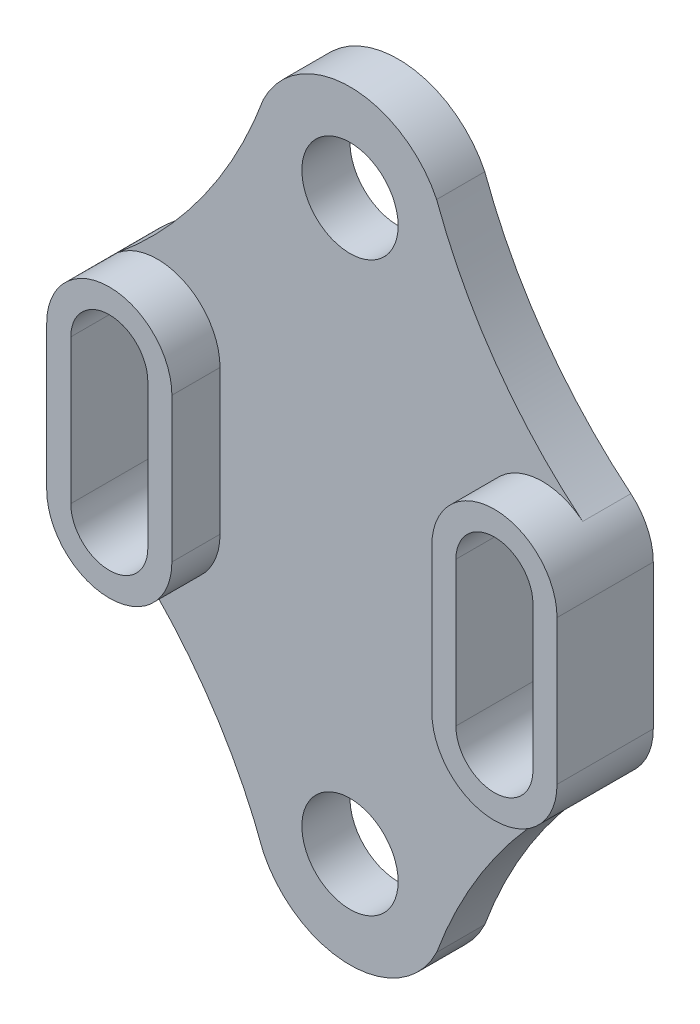
ISO-10303-21;
HEADER;
FILE_DESCRIPTION(('STEP AP214'),'2;1');
FILE_NAME('part.step','',(''),(''),'','','');
FILE_SCHEMA(('AUTOMOTIVE_DESIGN { 1 0 10303 214 1 1 1 1 }'));
ENDSEC;
DATA;
#1=APPLICATION_CONTEXT('core data for automotive mechanical design processes');
#2=APPLICATION_PROTOCOL_DEFINITION('international standard','automotive_design',2000,#1);
#3=PRODUCT_CONTEXT('',#1,'mechanical');
#4=PRODUCT('Part','Part','',(#3));
#5=PRODUCT_RELATED_PRODUCT_CATEGORY('part','',(#4));
#6=PRODUCT_DEFINITION_FORMATION('','',#4);
#7=PRODUCT_DEFINITION_CONTEXT('part definition',#1,'design');
#8=PRODUCT_DEFINITION('design','',#6,#7);
#9=PRODUCT_DEFINITION_SHAPE('','',#8);
#10=(LENGTH_UNIT() NAMED_UNIT(*) SI_UNIT(.MILLI.,.METRE.));
#11=(NAMED_UNIT(*) PLANE_ANGLE_UNIT() SI_UNIT($,.RADIAN.));
#12=(NAMED_UNIT(*) SI_UNIT($,.STERADIAN.) SOLID_ANGLE_UNIT());
#13=UNCERTAINTY_MEASURE_WITH_UNIT(LENGTH_MEASURE(1.E-05),#10,'distance_accuracy_value','');
#14=(GEOMETRIC_REPRESENTATION_CONTEXT(3) GLOBAL_UNCERTAINTY_ASSIGNED_CONTEXT((#13)) GLOBAL_UNIT_ASSIGNED_CONTEXT((#10,
#11,#12)) REPRESENTATION_CONTEXT('',''));
#15=CARTESIAN_POINT('',(0.,0.,0.));
#16=DIRECTION('',(0.,0.,1.));
#17=DIRECTION('',(1.,0.,0.));
#18=AXIS2_PLACEMENT_3D('',#15,#16,#17);
#19=CARTESIAN_POINT('',(0.,0.,10.));
#20=DIRECTION('',(0.,0.,1.));
#21=DIRECTION('',(1.,0.,0.));
#22=AXIS2_PLACEMENT_3D('',#19,#20,#21);
#23=PLANE('',#22);
#24=CARTESIAN_POINT('',(0.,-117.99999999991,10.));
#25=DIRECTION('',(0.,0.,1.));
#26=DIRECTION('',(1.,0.,0.));
#27=AXIS2_PLACEMENT_3D('',#24,#25,#26);
#28=CIRCLE('',#27,9.9999999999824);
#29=CARTESIAN_POINT('',(9.9999999999824,-117.99999999991,10.));
#30=VERTEX_POINT('',#29);
#31=EDGE_CURVE('E295',#30,#30,#28,.T.);
#32=ORIENTED_EDGE('',*,*,#31,.F.);
#33=EDGE_LOOP('',(#32));
#34=FACE_BOUND('',#33,.T.);
#35=CARTESIAN_POINT('',(0.,0.,10.));
#36=DIRECTION('',(0.,0.,1.));
#37=DIRECTION('',(1.,0.,0.));
#38=AXIS2_PLACEMENT_3D('',#35,#36,#37);
#39=CIRCLE('',#38,10.);
#40=CARTESIAN_POINT('',(10.,0.,10.));
#41=VERTEX_POINT('',#40);
#42=EDGE_CURVE('E301',#41,#41,#39,.T.);
#43=ORIENTED_EDGE('',*,*,#42,.F.);
#44=EDGE_LOOP('',(#43));
#45=FACE_BOUND('',#44,.T.);
#46=DIRECTION('',(0.,-1.,0.));
#47=VECTOR('',#46,1.);
#48=CARTESIAN_POINT('',(26.9999999996218,-43.9999999999274,10.));
#49=LINE('',#48,#47);
#50=CARTESIAN_POINT('',(26.9999999996218,-43.9999999999274,10.));
#51=VERTEX_POINT('',#50);
#52=CARTESIAN_POINT('',(26.9999999996218,-73.9999999999825,10.));
#53=VERTEX_POINT('',#52);
#54=EDGE_CURVE('E66',#51,#53,#49,.T.);
#55=ORIENTED_EDGE('',*,*,#54,.F.);
#56=CARTESIAN_POINT('',(39.9999999996218,-43.9999999999274,10.));
#57=DIRECTION('',(0.,0.,1.));
#58=DIRECTION('',(1.,0.,0.));
#59=AXIS2_PLACEMENT_3D('',#56,#57,#58);
#60=CIRCLE('',#59,13.);
#61=CARTESIAN_POINT('',(48.1941498448468,-33.9076311841338,10.));
#62=VERTEX_POINT('',#61);
#63=EDGE_CURVE('E255',#62,#51,#60,.T.);
#64=ORIENTED_EDGE('',*,*,#63,.F.);
#65=CARTESIAN_POINT('',(111.865980317354,43.2020180452665,10.));
#66=DIRECTION('',(0.,0.,1.));
#67=DIRECTION('',(1.,0.,0.));
#68=AXIS2_PLACEMENT_3D('',#65,#66,#67);
#69=CIRCLE('',#68,100.000000000004);
#70=CARTESIAN_POINT('',(17.9996405080933,8.71854010563166,10.));
#71=VERTEX_POINT('',#70);
#72=EDGE_CURVE('E386',#71,#62,#69,.T.);
#73=ORIENTED_EDGE('',*,*,#72,.F.);
#74=CARTESIAN_POINT('',(0.,0.,10.));
#75=DIRECTION('',(0.,0.,1.));
#76=DIRECTION('',(1.,0.,0.));
#77=AXIS2_PLACEMENT_3D('',#74,#75,#76);
#78=CIRCLE('',#77,19.9999999998526);
#79=CARTESIAN_POINT('',(-17.9996405080933,8.71854010563166,10.));
#80=VERTEX_POINT('',#79);
#81=EDGE_CURVE('E400',#71,#80,#78,.T.);
#82=ORIENTED_EDGE('',*,*,#81,.T.);
#83=CARTESIAN_POINT('',(-111.865980317354,43.2020180452665,10.));
#84=DIRECTION('',(0.,0.,1.));
#85=DIRECTION('',(1.,0.,0.));
#86=AXIS2_PLACEMENT_3D('',#83,#84,#85);
#87=CIRCLE('',#86,100.000000000004);
#88=CARTESIAN_POINT('',(-48.1941498448679,-33.9076311841512,10.));
#89=VERTEX_POINT('',#88);
#90=EDGE_CURVE('E360',#80,#89,#87,.F.);
#91=ORIENTED_EDGE('',*,*,#90,.T.);
#92=CARTESIAN_POINT('',(-39.9999999996218,-43.9999999999274,10.));
#93=DIRECTION('',(0.,0.,1.));
#94=DIRECTION('',(1.,0.,0.));
#95=AXIS2_PLACEMENT_3D('',#92,#93,#94);
#96=CIRCLE('',#95,13.);
#97=CARTESIAN_POINT('',(-26.9999999996218,-43.9999999999274,10.));
#98=VERTEX_POINT('',#97);
#99=EDGE_CURVE('E316',#98,#89,#96,.T.);
#100=ORIENTED_EDGE('',*,*,#99,.F.);
#101=DIRECTION('',(0.,1.,0.));
#102=VECTOR('',#101,1.);
#103=CARTESIAN_POINT('',(-26.9999999996218,-43.9999999999274,10.));
#104=LINE('',#103,#102);
#105=CARTESIAN_POINT('',(-26.9999999996218,-73.9999999999825,10.));
#106=VERTEX_POINT('',#105);
#107=EDGE_CURVE('E321',#106,#98,#104,.T.);
#108=ORIENTED_EDGE('',*,*,#107,.F.);
#109=CARTESIAN_POINT('',(-39.9999999996218,-73.9999999999825,10.));
#110=DIRECTION('',(0.,0.,1.));
#111=DIRECTION('',(1.,0.,0.));
#112=AXIS2_PLACEMENT_3D('',#109,#110,#111);
#113=CIRCLE('',#112,13.);
#114=CARTESIAN_POINT('',(-48.1941498448539,-84.0923688157703,10.));
#115=VERTEX_POINT('',#114);
#116=EDGE_CURVE('E11',#115,#106,#113,.T.);
#117=ORIENTED_EDGE('',*,*,#116,.F.);
#118=CARTESIAN_POINT('',(-111.865980317354,-161.202018045176,10.));
#119=DIRECTION('',(0.,0.,1.));
#120=DIRECTION('',(1.,0.,0.));
#121=AXIS2_PLACEMENT_3D('',#118,#119,#120);
#122=CIRCLE('',#121,100.000000000004);
#123=CARTESIAN_POINT('',(-17.9996405080933,-126.718540105542,10.));
#124=VERTEX_POINT('',#123);
#125=EDGE_CURVE('E459',#124,#115,#122,.T.);
#126=ORIENTED_EDGE('',*,*,#125,.F.);
#127=CARTESIAN_POINT('',(0.,-117.99999999991,10.));
#128=DIRECTION('',(0.,0.,1.));
#129=DIRECTION('',(1.,0.,0.));
#130=AXIS2_PLACEMENT_3D('',#127,#128,#129);
#131=CIRCLE('',#130,19.9999999998526);
#132=CARTESIAN_POINT('',(17.9996405080933,-126.718540105542,10.));
#133=VERTEX_POINT('',#132);
#134=EDGE_CURVE('E520',#124,#133,#131,.T.);
#135=ORIENTED_EDGE('',*,*,#134,.T.);
#136=CARTESIAN_POINT('',(111.865980317354,-161.202018045176,10.));
#137=DIRECTION('',(0.,0.,1.));
#138=DIRECTION('',(1.,0.,0.));
#139=AXIS2_PLACEMENT_3D('',#136,#137,#138);
#140=CIRCLE('',#139,100.000000000004);
#141=CARTESIAN_POINT('',(48.1941498448468,-84.0923688157761,10.));
#142=VERTEX_POINT('',#141);
#143=EDGE_CURVE('E397',#133,#142,#140,.F.);
#144=ORIENTED_EDGE('',*,*,#143,.T.);
#145=CARTESIAN_POINT('',(39.9999999996218,-73.9999999999825,10.));
#146=DIRECTION('',(0.,0.,1.));
#147=DIRECTION('',(1.,0.,0.));
#148=AXIS2_PLACEMENT_3D('',#145,#146,#147);
#149=CIRCLE('',#148,13.);
#150=EDGE_CURVE('E72',#53,#142,#149,.T.);
#151=ORIENTED_EDGE('',*,*,#150,.F.);
#152=EDGE_LOOP('',(#55,#64,#73,#82,#91,#100,#108,#117,#126,#135,#144,#151));
#153=FACE_BOUND('',#152,.T.);
#154=ADVANCED_FACE('F50',(#34,#45,#153),#23,.T.);
#155=CARTESIAN_POINT('',(0.,-117.99999999991,10.));
#156=DIRECTION('',(0.,0.,-1.));
#157=DIRECTION('',(-1.,0.,0.));
#158=AXIS2_PLACEMENT_3D('',#155,#156,#157);
#159=CYLINDRICAL_SURFACE('',#158,19.9999999998526);
#160=CARTESIAN_POINT('',(0.,-117.99999999991,0.));
#161=DIRECTION('',(0.,0.,1.));
#162=DIRECTION('',(1.,0.,0.));
#163=AXIS2_PLACEMENT_3D('',#160,#161,#162);
#164=CIRCLE('',#163,19.9999999998526);
#165=CARTESIAN_POINT('',(-17.9996405080933,-126.718540105542,0.));
#166=VERTEX_POINT('',#165);
#167=CARTESIAN_POINT('',(17.9996405080933,-126.718540105542,0.));
#168=VERTEX_POINT('',#167);
#169=EDGE_CURVE('E526',#166,#168,#164,.T.);
#170=ORIENTED_EDGE('',*,*,#169,.T.);
#171=DIRECTION('',(0.,0.,-1.));
#172=VECTOR('',#171,1.);
#173=CARTESIAN_POINT('',(17.9996405080933,-126.718540105542,10.));
#174=LINE('',#173,#172);
#175=EDGE_CURVE('E59',#133,#168,#174,.T.);
#176=ORIENTED_EDGE('',*,*,#175,.F.);
#177=ORIENTED_EDGE('',*,*,#134,.F.);
#178=DIRECTION('',(0.,0.,-1.));
#179=VECTOR('',#178,1.);
#180=CARTESIAN_POINT('',(-17.9996405080933,-126.718540105542,10.));
#181=LINE('',#180,#179);
#182=EDGE_CURVE('E464',#124,#166,#181,.T.);
#183=ORIENTED_EDGE('',*,*,#182,.T.);
#184=EDGE_LOOP('',(#170,#176,#177,#183));
#185=FACE_BOUND('',#184,.T.);
#186=ADVANCED_FACE('F47',(#185),#159,.T.);
#187=CARTESIAN_POINT('',(111.865980317354,-161.202018045176,10.));
#188=DIRECTION('',(0.,0.,-1.));
#189=DIRECTION('',(-1.,0.,0.));
#190=AXIS2_PLACEMENT_3D('',#187,#188,#189);
#191=CYLINDRICAL_SURFACE('',#190,100.000000000004);
#192=CARTESIAN_POINT('',(111.865980317354,-161.202018045176,0.));
#193=DIRECTION('',(0.,0.,1.));
#194=DIRECTION('',(1.,0.,0.));
#195=AXIS2_PLACEMENT_3D('',#192,#193,#194);
#196=CIRCLE('',#195,100.000000000004);
#197=CARTESIAN_POINT('',(48.341000131319,-83.971344784064,0.));
#198=VERTEX_POINT('',#197);
#199=EDGE_CURVE('E529',#168,#198,#196,.F.);
#200=ORIENTED_EDGE('',*,*,#199,.T.);
#201=DIRECTION('',(0.,0.,-1.));
#202=VECTOR('',#201,1.);
#203=CARTESIAN_POINT('',(48.341000131319,-83.971344784064,10.));
#204=LINE('',#203,#202);
#205=CARTESIAN_POINT('',(48.341000131319,-83.971344784064,10.));
#206=VERTEX_POINT('',#205);
#207=EDGE_CURVE('E440',#206,#198,#204,.T.);
#208=ORIENTED_EDGE('',*,*,#207,.F.);
#209=CARTESIAN_POINT('',(39.9999999996218,-73.9999999999825,10.));
#210=DIRECTION('',(0.,0.,1.));
#211=DIRECTION('',(0.630319218863457,-0.776336062753342,0.));
#212=AXIS2_PLACEMENT_3D('',#209,#210,#211);
#213=CIRCLE('',#212,13.);
#214=EDGE_CURVE('E287',#142,#206,#213,.T.);
#215=ORIENTED_EDGE('',*,*,#214,.F.);
#216=ORIENTED_EDGE('',*,*,#143,.F.);
#217=ORIENTED_EDGE('',*,*,#175,.T.);
#218=EDGE_LOOP('',(#200,#208,#215,#216,#217));
#219=FACE_BOUND('',#218,.T.);
#220=ADVANCED_FACE('F412',(#219),#191,.F.);
#221=CARTESIAN_POINT('',(39.9999999996218,-73.9999999999825,10.));
#222=DIRECTION('',(0.,0.,-1.));
#223=DIRECTION('',(-1.,0.,0.));
#224=AXIS2_PLACEMENT_3D('',#221,#222,#223);
#225=CYLINDRICAL_SURFACE('',#224,13.);
#226=CARTESIAN_POINT('',(39.9999999996218,-73.9999999999825,0.));
#227=DIRECTION('',(0.,0.,1.));
#228=DIRECTION('',(1.,0.,0.));
#229=AXIS2_PLACEMENT_3D('',#226,#227,#228);
#230=CIRCLE('',#229,13.);
#231=CARTESIAN_POINT('',(52.9999999996218,-73.9999999999825,0.));
#232=VERTEX_POINT('',#231);
#233=EDGE_CURVE('E535',#198,#232,#230,.T.);
#234=ORIENTED_EDGE('',*,*,#233,.T.);
#235=DIRECTION('',(0.,0.,-1.));
#236=VECTOR('',#235,1.);
#237=CARTESIAN_POINT('',(52.9999999996218,-73.9999999999825,10.));
#238=LINE('',#237,#236);
#239=CARTESIAN_POINT('',(52.9999999996218,-73.9999999999825,20.));
#240=VERTEX_POINT('',#239);
#241=EDGE_CURVE('E437',#240,#232,#238,.T.);
#242=ORIENTED_EDGE('',*,*,#241,.F.);
#243=CARTESIAN_POINT('',(39.9999999996218,-73.9999999999825,20.));
#244=DIRECTION('',(0.,0.,1.));
#245=DIRECTION('',(1.,0.,0.));
#246=AXIS2_PLACEMENT_3D('',#243,#244,#245);
#247=CIRCLE('',#246,13.);
#248=CARTESIAN_POINT('',(26.9999999996218,-73.9999999999825,20.));
#249=VERTEX_POINT('',#248);
#250=EDGE_CURVE('E257',#249,#240,#247,.T.);
#251=ORIENTED_EDGE('',*,*,#250,.F.);
#252=DIRECTION('',(0.,0.,-1.));
#253=VECTOR('',#252,1.);
#254=CARTESIAN_POINT('',(26.9999999996218,-73.9999999999825,20.));
#255=LINE('',#254,#253);
#256=EDGE_CURVE('E266',#249,#53,#255,.T.);
#257=ORIENTED_EDGE('',*,*,#256,.T.);
#258=ORIENTED_EDGE('',*,*,#150,.T.);
#259=ORIENTED_EDGE('',*,*,#214,.T.);
#260=ORIENTED_EDGE('',*,*,#207,.T.);
#261=EDGE_LOOP('',(#234,#242,#251,#257,#258,#259,#260));
#262=FACE_BOUND('',#261,.T.);
#263=ADVANCED_FACE('F425',(#262),#225,.T.);
#264=CARTESIAN_POINT('',(52.9999999996218,0.,10.));
#265=DIRECTION('',(-1.,0.,0.));
#266=DIRECTION('',(0.,-1.,0.));
#267=AXIS2_PLACEMENT_3D('',#264,#265,#266);
#268=PLANE('',#267);
#269=DIRECTION('',(0.,1.,0.));
#270=VECTOR('',#269,1.);
#271=CARTESIAN_POINT('',(52.9999999996218,0.,0.));
#272=LINE('',#271,#270);
#273=CARTESIAN_POINT('',(52.9999999996218,-43.9999999999274,0.));
#274=VERTEX_POINT('',#273);
#275=EDGE_CURVE('E506',#232,#274,#272,.T.);
#276=ORIENTED_EDGE('',*,*,#275,.T.);
#277=DIRECTION('',(0.,0.,-1.));
#278=VECTOR('',#277,1.);
#279=CARTESIAN_POINT('',(52.9999999996218,-43.9999999999274,10.));
#280=LINE('',#279,#278);
#281=CARTESIAN_POINT('',(52.9999999996218,-43.9999999999274,20.));
#282=VERTEX_POINT('',#281);
#283=EDGE_CURVE('E401',#282,#274,#280,.T.);
#284=ORIENTED_EDGE('',*,*,#283,.F.);
#285=DIRECTION('',(0.,1.,0.));
#286=VECTOR('',#285,1.);
#287=CARTESIAN_POINT('',(52.9999999996218,-73.9999999999825,20.));
#288=LINE('',#287,#286);
#289=EDGE_CURVE('E263',#240,#282,#288,.T.);
#290=ORIENTED_EDGE('',*,*,#289,.F.);
#291=ORIENTED_EDGE('',*,*,#241,.T.);
#292=EDGE_LOOP('',(#276,#284,#290,#291));
#293=FACE_BOUND('',#292,.T.);
#294=ADVANCED_FACE('F422',(#293),#268,.F.);
#295=CARTESIAN_POINT('',(39.9999999996218,-43.9999999999274,10.));
#296=DIRECTION('',(0.,0.,-1.));
#297=DIRECTION('',(-1.,0.,0.));
#298=AXIS2_PLACEMENT_3D('',#295,#296,#297);
#299=CYLINDRICAL_SURFACE('',#298,13.);
#300=CARTESIAN_POINT('',(39.9999999996218,-43.9999999999274,0.));
#301=DIRECTION('',(0.,0.,1.));
#302=DIRECTION('',(1.,0.,0.));
#303=AXIS2_PLACEMENT_3D('',#300,#301,#302);
#304=CIRCLE('',#303,13.);
#305=CARTESIAN_POINT('',(48.341000131319,-34.0286552158459,0.));
#306=VERTEX_POINT('',#305);
#307=EDGE_CURVE('E501',#274,#306,#304,.T.);
#308=ORIENTED_EDGE('',*,*,#307,.T.);
#309=DIRECTION('',(0.,0.,-1.));
#310=VECTOR('',#309,1.);
#311=CARTESIAN_POINT('',(48.341000131319,-34.0286552158459,10.));
#312=LINE('',#311,#310);
#313=CARTESIAN_POINT('',(48.341000131319,-34.0286552158459,10.));
#314=VERTEX_POINT('',#313);
#315=EDGE_CURVE('E402',#314,#306,#312,.T.);
#316=ORIENTED_EDGE('',*,*,#315,.F.);
#317=CARTESIAN_POINT('',(39.9999999996218,-43.9999999999274,10.));
#318=DIRECTION('',(0.,0.,1.));
#319=DIRECTION('',(0.641615394745934,0.767026521852419,0.));
#320=AXIS2_PLACEMENT_3D('',#317,#318,#319);
#321=CIRCLE('',#320,13.);
#322=EDGE_CURVE('E281',#314,#62,#321,.T.);
#323=ORIENTED_EDGE('',*,*,#322,.T.);
#324=ORIENTED_EDGE('',*,*,#63,.T.);
#325=DIRECTION('',(0.,0.,-1.));
#326=VECTOR('',#325,1.);
#327=CARTESIAN_POINT('',(26.9999999996218,-43.9999999999274,20.));
#328=LINE('',#327,#326);
#329=CARTESIAN_POINT('',(26.9999999996218,-43.9999999999274,20.));
#330=VERTEX_POINT('',#329);
#331=EDGE_CURVE('E272',#330,#51,#328,.T.);
#332=ORIENTED_EDGE('',*,*,#331,.F.);
#333=CARTESIAN_POINT('',(39.9999999996218,-43.9999999999274,20.));
#334=DIRECTION('',(0.,0.,1.));
#335=DIRECTION('',(1.,0.,0.));
#336=AXIS2_PLACEMENT_3D('',#333,#334,#335);
#337=CIRCLE('',#336,13.);
#338=EDGE_CURVE('E254',#282,#330,#337,.T.);
#339=ORIENTED_EDGE('',*,*,#338,.F.);
#340=ORIENTED_EDGE('',*,*,#283,.T.);
#341=EDGE_LOOP('',(#308,#316,#323,#324,#332,#339,#340));
#342=FACE_BOUND('',#341,.T.);
#343=ADVANCED_FACE('F377',(#342),#299,.T.);
#344=CARTESIAN_POINT('',(111.865980317354,43.2020180452665,10.));
#345=DIRECTION('',(0.,0.,-1.));
#346=DIRECTION('',(-1.,0.,0.));
#347=AXIS2_PLACEMENT_3D('',#344,#345,#346);
#348=CYLINDRICAL_SURFACE('',#347,100.000000000004);
#349=CARTESIAN_POINT('',(111.865980317354,43.2020180452665,0.));
#350=DIRECTION('',(0.,0.,1.));
#351=DIRECTION('',(1.,0.,0.));
#352=AXIS2_PLACEMENT_3D('',#349,#350,#351);
#353=CIRCLE('',#352,100.000000000004);
#354=CARTESIAN_POINT('',(17.9996405080933,8.71854010563166,0.));
#355=VERTEX_POINT('',#354);
#356=EDGE_CURVE('E496',#355,#306,#353,.T.);
#357=ORIENTED_EDGE('',*,*,#356,.F.);
#358=DIRECTION('',(0.,0.,-1.));
#359=VECTOR('',#358,1.);
#360=CARTESIAN_POINT('',(17.9996405080933,8.71854010563166,10.));
#361=LINE('',#360,#359);
#362=EDGE_CURVE('E404',#71,#355,#361,.T.);
#363=ORIENTED_EDGE('',*,*,#362,.F.);
#364=ORIENTED_EDGE('',*,*,#72,.T.);
#365=ORIENTED_EDGE('',*,*,#322,.F.);
#366=ORIENTED_EDGE('',*,*,#315,.T.);
#367=EDGE_LOOP('',(#357,#363,#364,#365,#366));
#368=FACE_BOUND('',#367,.T.);
#369=ADVANCED_FACE('F374',(#368),#348,.F.);
#370=CARTESIAN_POINT('',(0.,0.,10.));
#371=DIRECTION('',(0.,0.,-1.));
#372=DIRECTION('',(-1.,0.,0.));
#373=AXIS2_PLACEMENT_3D('',#370,#371,#372);
#374=CYLINDRICAL_SURFACE('',#373,19.9999999998526);
#375=CARTESIAN_POINT('',(0.,0.,0.));
#376=DIRECTION('',(0.,0.,1.));
#377=DIRECTION('',(1.,0.,0.));
#378=AXIS2_PLACEMENT_3D('',#375,#376,#377);
#379=CIRCLE('',#378,19.9999999998526);
#380=CARTESIAN_POINT('',(-17.9996405080933,8.71854010563166,0.));
#381=VERTEX_POINT('',#380);
#382=EDGE_CURVE('E491',#355,#381,#379,.T.);
#383=ORIENTED_EDGE('',*,*,#382,.T.);
#384=DIRECTION('',(0.,0.,-1.));
#385=VECTOR('',#384,1.);
#386=CARTESIAN_POINT('',(-17.9996405080933,8.71854010563166,10.));
#387=LINE('',#386,#385);
#388=EDGE_CURVE('E486',#80,#381,#387,.T.);
#389=ORIENTED_EDGE('',*,*,#388,.F.);
#390=ORIENTED_EDGE('',*,*,#81,.F.);
#391=ORIENTED_EDGE('',*,*,#362,.T.);
#392=EDGE_LOOP('',(#383,#389,#390,#391));
#393=FACE_BOUND('',#392,.T.);
#394=ADVANCED_FACE('F367',(#393),#374,.T.);
#395=CARTESIAN_POINT('',(-111.865980317354,43.2020180452665,10.));
#396=DIRECTION('',(0.,0.,-1.));
#397=DIRECTION('',(-1.,0.,0.));
#398=AXIS2_PLACEMENT_3D('',#395,#396,#397);
#399=CYLINDRICAL_SURFACE('',#398,100.000000000004);
#400=CARTESIAN_POINT('',(-111.865980317354,43.2020180452665,0.));
#401=DIRECTION('',(0.,0.,1.));
#402=DIRECTION('',(1.,0.,0.));
#403=AXIS2_PLACEMENT_3D('',#400,#401,#402);
#404=CIRCLE('',#403,100.000000000004);
#405=CARTESIAN_POINT('',(-48.341000131319,-34.0286552158459,0.));
#406=VERTEX_POINT('',#405);
#407=EDGE_CURVE('E502',#381,#406,#404,.F.);
#408=ORIENTED_EDGE('',*,*,#407,.T.);
#409=DIRECTION('',(0.,0.,-1.));
#410=VECTOR('',#409,1.);
#411=CARTESIAN_POINT('',(-48.341000131319,-34.0286552158459,10.));
#412=LINE('',#411,#410);
#413=CARTESIAN_POINT('',(-48.341000131319,-34.0286552158459,10.));
#414=VERTEX_POINT('',#413);
#415=EDGE_CURVE('E484',#414,#406,#412,.T.);
#416=ORIENTED_EDGE('',*,*,#415,.F.);
#417=CARTESIAN_POINT('',(-39.9999999996218,-43.9999999999274,10.));
#418=DIRECTION('',(0.,0.,1.));
#419=DIRECTION('',(-0.63031921886509,0.776336062752016,0.));
#420=AXIS2_PLACEMENT_3D('',#417,#418,#419);
#421=CIRCLE('',#420,13.);
#422=EDGE_CURVE('E352',#89,#414,#421,.T.);
#423=ORIENTED_EDGE('',*,*,#422,.F.);
#424=ORIENTED_EDGE('',*,*,#90,.F.);
#425=ORIENTED_EDGE('',*,*,#388,.T.);
#426=EDGE_LOOP('',(#408,#416,#423,#424,#425));
#427=FACE_BOUND('',#426,.T.);
#428=ADVANCED_FACE('F358',(#427),#399,.F.);
#429=CARTESIAN_POINT('',(-39.9999999996218,-43.9999999999274,10.));
#430=DIRECTION('',(0.,0.,-1.));
#431=DIRECTION('',(-1.,0.,0.));
#432=AXIS2_PLACEMENT_3D('',#429,#430,#431);
#433=CYLINDRICAL_SURFACE('',#432,13.);
#434=CARTESIAN_POINT('',(-39.9999999996218,-43.9999999999274,0.));
#435=DIRECTION('',(0.,0.,1.));
#436=DIRECTION('',(1.,0.,0.));
#437=AXIS2_PLACEMENT_3D('',#434,#435,#436);
#438=CIRCLE('',#437,13.);
#439=CARTESIAN_POINT('',(-52.9999999996218,-43.9999999999274,0.));
#440=VERTEX_POINT('',#439);
#441=EDGE_CURVE('E512',#406,#440,#438,.T.);
#442=ORIENTED_EDGE('',*,*,#441,.T.);
#443=DIRECTION('',(0.,0.,-1.));
#444=VECTOR('',#443,1.);
#445=CARTESIAN_POINT('',(-52.9999999996218,-43.9999999999274,10.));
#446=LINE('',#445,#444);
#447=CARTESIAN_POINT('',(-52.9999999996218,-43.9999999999274,20.));
#448=VERTEX_POINT('',#447);
#449=EDGE_CURVE('E472',#448,#440,#446,.T.);
#450=ORIENTED_EDGE('',*,*,#449,.F.);
#451=CARTESIAN_POINT('',(-39.9999999996218,-43.9999999999274,20.));
#452=DIRECTION('',(0.,0.,1.));
#453=DIRECTION('',(1.,0.,0.));
#454=AXIS2_PLACEMENT_3D('',#451,#452,#453);
#455=CIRCLE('',#454,13.);
#456=CARTESIAN_POINT('',(-26.9999999996218,-43.9999999999274,20.));
#457=VERTEX_POINT('',#456);
#458=EDGE_CURVE('E320',#457,#448,#455,.T.);
#459=ORIENTED_EDGE('',*,*,#458,.F.);
#460=DIRECTION('',(0.,0.,-1.));
#461=VECTOR('',#460,1.);
#462=CARTESIAN_POINT('',(-26.9999999996218,-43.9999999999274,20.));
#463=LINE('',#462,#461);
#464=EDGE_CURVE('E327',#457,#98,#463,.T.);
#465=ORIENTED_EDGE('',*,*,#464,.T.);
#466=ORIENTED_EDGE('',*,*,#99,.T.);
#467=ORIENTED_EDGE('',*,*,#422,.T.);
#468=ORIENTED_EDGE('',*,*,#415,.T.);
#469=EDGE_LOOP('',(#442,#450,#459,#465,#466,#467,#468));
#470=FACE_BOUND('',#469,.T.);
#471=ADVANCED_FACE('F369',(#470),#433,.T.);
#472=CARTESIAN_POINT('',(-52.9999999996218,0.,10.));
#473=DIRECTION('',(1.,0.,0.));
#474=DIRECTION('',(0.,1.,0.));
#475=AXIS2_PLACEMENT_3D('',#472,#473,#474);
#476=PLANE('',#475);
#477=DIRECTION('',(0.,-1.,0.));
#478=VECTOR('',#477,1.);
#479=CARTESIAN_POINT('',(-52.9999999996218,0.,0.));
#480=LINE('',#479,#478);
#481=CARTESIAN_POINT('',(-52.9999999996218,-73.9999999999825,0.));
#482=VERTEX_POINT('',#481);
#483=EDGE_CURVE('E511',#440,#482,#480,.T.);
#484=ORIENTED_EDGE('',*,*,#483,.T.);
#485=DIRECTION('',(0.,0.,-1.));
#486=VECTOR('',#485,1.);
#487=CARTESIAN_POINT('',(-52.9999999996218,-73.9999999999825,10.));
#488=LINE('',#487,#486);
#489=CARTESIAN_POINT('',(-52.9999999996218,-73.9999999999825,20.));
#490=VERTEX_POINT('',#489);
#491=EDGE_CURVE('E466',#490,#482,#488,.T.);
#492=ORIENTED_EDGE('',*,*,#491,.F.);
#493=DIRECTION('',(0.,-1.,0.));
#494=VECTOR('',#493,1.);
#495=CARTESIAN_POINT('',(-52.9999999996218,-73.9999999999825,20.));
#496=LINE('',#495,#494);
#497=EDGE_CURVE('E319',#448,#490,#496,.T.);
#498=ORIENTED_EDGE('',*,*,#497,.F.);
#499=ORIENTED_EDGE('',*,*,#449,.T.);
#500=EDGE_LOOP('',(#484,#492,#498,#499));
#501=FACE_BOUND('',#500,.T.);
#502=ADVANCED_FACE('F559',(#501),#476,.F.);
#503=CARTESIAN_POINT('',(-39.9999999996218,-73.9999999999825,10.));
#504=DIRECTION('',(0.,0.,-1.));
#505=DIRECTION('',(-1.,0.,0.));
#506=AXIS2_PLACEMENT_3D('',#503,#504,#505);
#507=CYLINDRICAL_SURFACE('',#506,13.);
#508=CARTESIAN_POINT('',(-39.9999999996218,-73.9999999999825,0.));
#509=DIRECTION('',(0.,0.,1.));
#510=DIRECTION('',(1.,0.,0.));
#511=AXIS2_PLACEMENT_3D('',#508,#509,#510);
#512=CIRCLE('',#511,13.);
#513=CARTESIAN_POINT('',(-48.3410001313181,-83.9713447840648,0.));
#514=VERTEX_POINT('',#513);
#515=EDGE_CURVE('E514',#482,#514,#512,.T.);
#516=ORIENTED_EDGE('',*,*,#515,.T.);
#517=DIRECTION('',(0.,0.,-1.));
#518=VECTOR('',#517,1.);
#519=CARTESIAN_POINT('',(-48.3410001313181,-83.9713447840648,10.));
#520=LINE('',#519,#518);
#521=CARTESIAN_POINT('',(-48.3410001313181,-83.9713447840648,10.));
#522=VERTEX_POINT('',#521);
#523=EDGE_CURVE('E463',#522,#514,#520,.T.);
#524=ORIENTED_EDGE('',*,*,#523,.F.);
#525=CARTESIAN_POINT('',(-111.865980317354,-161.202018045176,10.));
#526=DIRECTION('',(0.,0.,1.));
#527=DIRECTION('',(0.636718304724972,0.771096492294031,0.));
#528=AXIS2_PLACEMENT_3D('',#525,#526,#527);
#529=CIRCLE('',#528,100.000000000004);
#530=EDGE_CURVE('E465',#115,#522,#529,.T.);
#531=ORIENTED_EDGE('',*,*,#530,.F.);
#532=ORIENTED_EDGE('',*,*,#116,.T.);
#533=DIRECTION('',(0.,0.,-1.));
#534=VECTOR('',#533,1.);
#535=CARTESIAN_POINT('',(-26.9999999996218,-73.9999999999825,20.));
#536=LINE('',#535,#534);
#537=CARTESIAN_POINT('',(-26.9999999996218,-73.9999999999825,20.));
#538=VERTEX_POINT('',#537);
#539=EDGE_CURVE('E334',#538,#106,#536,.T.);
#540=ORIENTED_EDGE('',*,*,#539,.F.);
#541=CARTESIAN_POINT('',(-39.9999999996218,-73.9999999999825,20.));
#542=DIRECTION('',(0.,0.,1.));
#543=DIRECTION('',(1.,0.,0.));
#544=AXIS2_PLACEMENT_3D('',#541,#542,#543);
#545=CIRCLE('',#544,13.);
#546=EDGE_CURVE('E322',#490,#538,#545,.T.);
#547=ORIENTED_EDGE('',*,*,#546,.F.);
#548=ORIENTED_EDGE('',*,*,#491,.T.);
#549=EDGE_LOOP('',(#516,#524,#531,#532,#540,#547,#548));
#550=FACE_BOUND('',#549,.T.);
#551=ADVANCED_FACE('F551',(#550),#507,.T.);
#552=CARTESIAN_POINT('',(-111.865980317354,-161.202018045176,10.));
#553=DIRECTION('',(0.,0.,-1.));
#554=DIRECTION('',(-1.,0.,0.));
#555=AXIS2_PLACEMENT_3D('',#552,#553,#554);
#556=CYLINDRICAL_SURFACE('',#555,100.000000000004);
#557=CARTESIAN_POINT('',(-111.865980317354,-161.202018045176,0.));
#558=DIRECTION('',(0.,0.,1.));
#559=DIRECTION('',(1.,0.,0.));
#560=AXIS2_PLACEMENT_3D('',#557,#558,#559);
#561=CIRCLE('',#560,100.000000000004);
#562=EDGE_CURVE('E477',#166,#514,#561,.T.);
#563=ORIENTED_EDGE('',*,*,#562,.F.);
#564=ORIENTED_EDGE('',*,*,#182,.F.);
#565=ORIENTED_EDGE('',*,*,#125,.T.);
#566=ORIENTED_EDGE('',*,*,#530,.T.);
#567=ORIENTED_EDGE('',*,*,#523,.T.);
#568=EDGE_LOOP('',(#563,#564,#565,#566,#567));
#569=FACE_BOUND('',#568,.T.);
#570=ADVANCED_FACE('F548',(#569),#556,.F.);
#571=CARTESIAN_POINT('',(0.,0.,0.));
#572=DIRECTION('',(0.,0.,1.));
#573=DIRECTION('',(1.,0.,0.));
#574=AXIS2_PLACEMENT_3D('',#571,#572,#573);
#575=PLANE('',#574);
#576=CARTESIAN_POINT('',(0.,0.,0.));
#577=DIRECTION('',(0.,0.,1.));
#578=DIRECTION('',(1.,0.,0.));
#579=AXIS2_PLACEMENT_3D('',#576,#577,#578);
#580=CIRCLE('',#579,10.);
#581=CARTESIAN_POINT('',(10.,0.,0.));
#582=VERTEX_POINT('',#581);
#583=EDGE_CURVE('E277',#582,#582,#580,.T.);
#584=ORIENTED_EDGE('',*,*,#583,.T.);
#585=EDGE_LOOP('',(#584));
#586=FACE_BOUND('',#585,.T.);
#587=CARTESIAN_POINT('',(0.,-117.99999999991,0.));
#588=DIRECTION('',(0.,0.,1.));
#589=DIRECTION('',(1.,0.,0.));
#590=AXIS2_PLACEMENT_3D('',#587,#588,#589);
#591=CIRCLE('',#590,9.9999999999824);
#592=CARTESIAN_POINT('',(9.9999999999824,-117.99999999991,0.));
#593=VERTEX_POINT('',#592);
#594=EDGE_CURVE('E297',#593,#593,#591,.T.);
#595=ORIENTED_EDGE('',*,*,#594,.T.);
#596=EDGE_LOOP('',(#595));
#597=FACE_BOUND('',#596,.T.);
#598=DIRECTION('',(0.,1.,0.));
#599=VECTOR('',#598,1.);
#600=CARTESIAN_POINT('',(47.9999999989875,-73.9999999999825,0.));
#601=LINE('',#600,#599);
#602=CARTESIAN_POINT('',(47.9999999989875,-73.9999999999825,0.));
#603=VERTEX_POINT('',#602);
#604=CARTESIAN_POINT('',(47.9999999989875,-43.9999999999274,0.));
#605=VERTEX_POINT('',#604);
#606=EDGE_CURVE('E237',#603,#605,#601,.T.);
#607=ORIENTED_EDGE('',*,*,#606,.T.);
#608=CARTESIAN_POINT('',(39.9999999996218,-43.9999999999274,0.));
#609=DIRECTION('',(0.,0.,1.));
#610=DIRECTION('',(1.,0.,0.));
#611=AXIS2_PLACEMENT_3D('',#608,#609,#610);
#612=CIRCLE('',#611,7.99999999936566);
#613=CARTESIAN_POINT('',(32.0000000002561,-43.9999999999274,0.));
#614=VERTEX_POINT('',#613);
#615=EDGE_CURVE('E338',#605,#614,#612,.T.);
#616=ORIENTED_EDGE('',*,*,#615,.T.);
#617=DIRECTION('',(0.,-1.,0.));
#618=VECTOR('',#617,1.);
#619=CARTESIAN_POINT('',(32.0000000002561,-43.9999999999274,0.));
#620=LINE('',#619,#618);
#621=CARTESIAN_POINT('',(32.0000000002561,-73.9999999999825,0.));
#622=VERTEX_POINT('',#621);
#623=EDGE_CURVE('E231',#614,#622,#620,.T.);
#624=ORIENTED_EDGE('',*,*,#623,.T.);
#625=CARTESIAN_POINT('',(39.9999999996218,-73.9999999999825,0.));
#626=DIRECTION('',(0.,0.,1.));
#627=DIRECTION('',(1.,0.,0.));
#628=AXIS2_PLACEMENT_3D('',#625,#626,#627);
#629=CIRCLE('',#628,7.99999999936566);
#630=EDGE_CURVE('E997',#622,#603,#629,.T.);
#631=ORIENTED_EDGE('',*,*,#630,.T.);
#632=EDGE_LOOP('',(#607,#616,#624,#631));
#633=FACE_BOUND('',#632,.T.);
#634=DIRECTION('',(0.,1.,0.));
#635=VECTOR('',#634,1.);
#636=CARTESIAN_POINT('',(-32.0000000002561,-73.9999999999825,0.));
#637=LINE('',#636,#635);
#638=CARTESIAN_POINT('',(-32.0000000002561,-73.9999999999825,0.));
#639=VERTEX_POINT('',#638);
#640=CARTESIAN_POINT('',(-32.0000000002561,-43.9999999999274,0.));
#641=VERTEX_POINT('',#640);
#642=EDGE_CURVE('E974',#639,#641,#637,.T.);
#643=ORIENTED_EDGE('',*,*,#642,.T.);
#644=CARTESIAN_POINT('',(-39.9999999996218,-43.9999999999274,0.));
#645=DIRECTION('',(0.,0.,1.));
#646=DIRECTION('',(1.,0.,0.));
#647=AXIS2_PLACEMENT_3D('',#644,#645,#646);
#648=CIRCLE('',#647,7.99999999936566);
#649=CARTESIAN_POINT('',(-47.9999999989875,-43.9999999999274,0.));
#650=VERTEX_POINT('',#649);
#651=EDGE_CURVE('E337',#641,#650,#648,.T.);
#652=ORIENTED_EDGE('',*,*,#651,.T.);
#653=DIRECTION('',(0.,-1.,0.));
#654=VECTOR('',#653,1.);
#655=CARTESIAN_POINT('',(-47.9999999989875,-43.9999999999274,0.));
#656=LINE('',#655,#654);
#657=CARTESIAN_POINT('',(-47.9999999989874,-73.9999999999825,0.));
#658=VERTEX_POINT('',#657);
#659=EDGE_CURVE('E969',#650,#658,#656,.T.);
#660=ORIENTED_EDGE('',*,*,#659,.T.);
#661=CARTESIAN_POINT('',(-39.9999999996218,-73.9999999999825,0.));
#662=DIRECTION('',(0.,0.,1.));
#663=DIRECTION('',(1.,0.,0.));
#664=AXIS2_PLACEMENT_3D('',#661,#662,#663);
#665=CIRCLE('',#664,7.99999999936565);
#666=EDGE_CURVE('E981',#658,#639,#665,.T.);
#667=ORIENTED_EDGE('',*,*,#666,.T.);
#668=EDGE_LOOP('',(#643,#652,#660,#667));
#669=FACE_BOUND('',#668,.T.);
#670=ORIENTED_EDGE('',*,*,#169,.F.);
#671=ORIENTED_EDGE('',*,*,#562,.T.);
#672=ORIENTED_EDGE('',*,*,#515,.F.);
#673=ORIENTED_EDGE('',*,*,#483,.F.);
#674=ORIENTED_EDGE('',*,*,#441,.F.);
#675=ORIENTED_EDGE('',*,*,#407,.F.);
#676=ORIENTED_EDGE('',*,*,#382,.F.);
#677=ORIENTED_EDGE('',*,*,#356,.T.);
#678=ORIENTED_EDGE('',*,*,#307,.F.);
#679=ORIENTED_EDGE('',*,*,#275,.F.);
#680=ORIENTED_EDGE('',*,*,#233,.F.);
#681=ORIENTED_EDGE('',*,*,#199,.F.);
#682=EDGE_LOOP('',(#670,#671,#672,#673,#674,#675,#676,#677,#678,#679,#680,#681));
#683=FACE_BOUND('',#682,.T.);
#684=ADVANCED_FACE('F500',(#586,#597,#633,#669,#683),#575,.F.);
#685=CARTESIAN_POINT('',(-39.9999999996218,-43.9999999999274,0.));
#686=DIRECTION('',(0.,0.,1.));
#687=DIRECTION('',(1.,0.,0.));
#688=AXIS2_PLACEMENT_3D('',#685,#686,#687);
#689=CYLINDRICAL_SURFACE('',#688,7.99999999936566);
#690=DIRECTION('',(0.,0.,1.));
#691=VECTOR('',#690,1.);
#692=CARTESIAN_POINT('',(-32.0000000002561,-43.9999999999274,0.));
#693=LINE('',#692,#691);
#694=CARTESIAN_POINT('',(-32.0000000002561,-43.9999999999274,20.));
#695=VERTEX_POINT('',#694);
#696=EDGE_CURVE('E976',#641,#695,#693,.T.);
#697=ORIENTED_EDGE('',*,*,#696,.T.);
#698=CARTESIAN_POINT('',(-39.9999999996218,-43.9999999999274,20.));
#699=DIRECTION('',(0.,0.,1.));
#700=DIRECTION('',(1.,0.,0.));
#701=AXIS2_PLACEMENT_3D('',#698,#699,#700);
#702=CIRCLE('',#701,7.99999999936566);
#703=CARTESIAN_POINT('',(-47.9999999989875,-43.9999999999274,20.));
#704=VERTEX_POINT('',#703);
#705=EDGE_CURVE('E303',#695,#704,#702,.T.);
#706=ORIENTED_EDGE('',*,*,#705,.T.);
#707=DIRECTION('',(0.,0.,1.));
#708=VECTOR('',#707,1.);
#709=CARTESIAN_POINT('',(-47.9999999989875,-43.9999999999274,0.));
#710=LINE('',#709,#708);
#711=EDGE_CURVE('E524',#650,#704,#710,.T.);
#712=ORIENTED_EDGE('',*,*,#711,.F.);
#713=ORIENTED_EDGE('',*,*,#651,.F.);
#714=EDGE_LOOP('',(#697,#706,#712,#713));
#715=FACE_BOUND('',#714,.T.);
#716=ADVANCED_FACE('F546',(#715),#689,.F.);
#717=CARTESIAN_POINT('',(-32.0000000002561,-73.9999999999825,0.));
#718=DIRECTION('',(1.,0.,0.));
#719=DIRECTION('',(0.,0.,-1.));
#720=AXIS2_PLACEMENT_3D('',#717,#718,#719);
#721=PLANE('',#720);
#722=DIRECTION('',(0.,0.,1.));
#723=VECTOR('',#722,1.);
#724=CARTESIAN_POINT('',(-32.0000000002561,-73.9999999999825,0.));
#725=LINE('',#724,#723);
#726=CARTESIAN_POINT('',(-32.0000000002561,-73.9999999999825,20.));
#727=VERTEX_POINT('',#726);
#728=EDGE_CURVE('E978',#639,#727,#725,.T.);
#729=ORIENTED_EDGE('',*,*,#728,.T.);
#730=DIRECTION('',(0.,1.,0.));
#731=VECTOR('',#730,1.);
#732=CARTESIAN_POINT('',(-32.0000000002561,-43.9999999999274,20.));
#733=LINE('',#732,#731);
#734=EDGE_CURVE('E311',#727,#695,#733,.T.);
#735=ORIENTED_EDGE('',*,*,#734,.T.);
#736=ORIENTED_EDGE('',*,*,#696,.F.);
#737=ORIENTED_EDGE('',*,*,#642,.F.);
#738=EDGE_LOOP('',(#729,#735,#736,#737));
#739=FACE_BOUND('',#738,.T.);
#740=ADVANCED_FACE('F825',(#739),#721,.F.);
#741=CARTESIAN_POINT('',(-39.9999999996218,-73.9999999999825,0.));
#742=DIRECTION('',(0.,0.,1.));
#743=DIRECTION('',(1.,0.,0.));
#744=AXIS2_PLACEMENT_3D('',#741,#742,#743);
#745=CYLINDRICAL_SURFACE('',#744,7.99999999936565);
#746=DIRECTION('',(0.,0.,1.));
#747=VECTOR('',#746,1.);
#748=CARTESIAN_POINT('',(-47.9999999989874,-73.9999999999825,0.));
#749=LINE('',#748,#747);
#750=CARTESIAN_POINT('',(-47.9999999989874,-73.9999999999825,20.));
#751=VERTEX_POINT('',#750);
#752=EDGE_CURVE('E971',#658,#751,#749,.T.);
#753=ORIENTED_EDGE('',*,*,#752,.T.);
#754=CARTESIAN_POINT('',(-39.9999999996218,-73.9999999999825,20.));
#755=DIRECTION('',(0.,0.,1.));
#756=DIRECTION('',(1.,0.,0.));
#757=AXIS2_PLACEMENT_3D('',#754,#755,#756);
#758=CIRCLE('',#757,7.99999999936565);
#759=EDGE_CURVE('E309',#751,#727,#758,.T.);
#760=ORIENTED_EDGE('',*,*,#759,.T.);
#761=ORIENTED_EDGE('',*,*,#728,.F.);
#762=ORIENTED_EDGE('',*,*,#666,.F.);
#763=EDGE_LOOP('',(#753,#760,#761,#762));
#764=FACE_BOUND('',#763,.T.);
#765=ADVANCED_FACE('F835',(#764),#745,.F.);
#766=CARTESIAN_POINT('',(-47.9999999989875,-43.9999999999274,0.));
#767=DIRECTION('',(-1.,0.,0.));
#768=DIRECTION('',(0.,-1.,0.));
#769=AXIS2_PLACEMENT_3D('',#766,#767,#768);
#770=PLANE('',#769);
#771=ORIENTED_EDGE('',*,*,#711,.T.);
#772=DIRECTION('',(0.,-1.,0.));
#773=VECTOR('',#772,1.);
#774=CARTESIAN_POINT('',(-47.9999999989875,-43.9999999999274,20.));
#775=LINE('',#774,#773);
#776=EDGE_CURVE('E307',#704,#751,#775,.T.);
#777=ORIENTED_EDGE('',*,*,#776,.T.);
#778=ORIENTED_EDGE('',*,*,#752,.F.);
#779=ORIENTED_EDGE('',*,*,#659,.F.);
#780=EDGE_LOOP('',(#771,#777,#778,#779));
#781=FACE_BOUND('',#780,.T.);
#782=ADVANCED_FACE('F638',(#781),#770,.F.);
#783=CARTESIAN_POINT('',(39.9999999996218,-43.9999999999274,0.));
#784=DIRECTION('',(0.,0.,1.));
#785=DIRECTION('',(1.,0.,0.));
#786=AXIS2_PLACEMENT_3D('',#783,#784,#785);
#787=CYLINDRICAL_SURFACE('',#786,7.99999999936566);
#788=DIRECTION('',(0.,0.,1.));
#789=VECTOR('',#788,1.);
#790=CARTESIAN_POINT('',(47.9999999989875,-43.9999999999274,0.));
#791=LINE('',#790,#789);
#792=CARTESIAN_POINT('',(47.9999999989875,-43.9999999999274,20.));
#793=VERTEX_POINT('',#792);
#794=EDGE_CURVE('E242',#605,#793,#791,.T.);
#795=ORIENTED_EDGE('',*,*,#794,.T.);
#796=CARTESIAN_POINT('',(39.9999999996218,-43.9999999999274,20.));
#797=DIRECTION('',(0.,0.,1.));
#798=DIRECTION('',(1.,0.,0.));
#799=AXIS2_PLACEMENT_3D('',#796,#797,#798);
#800=CIRCLE('',#799,7.99999999936566);
#801=CARTESIAN_POINT('',(32.0000000002561,-43.9999999999274,20.));
#802=VERTEX_POINT('',#801);
#803=EDGE_CURVE('E239',#793,#802,#800,.T.);
#804=ORIENTED_EDGE('',*,*,#803,.T.);
#805=DIRECTION('',(0.,0.,1.));
#806=VECTOR('',#805,1.);
#807=CARTESIAN_POINT('',(32.0000000002561,-43.9999999999274,0.));
#808=LINE('',#807,#806);
#809=EDGE_CURVE('E224',#614,#802,#808,.T.);
#810=ORIENTED_EDGE('',*,*,#809,.F.);
#811=ORIENTED_EDGE('',*,*,#615,.F.);
#812=EDGE_LOOP('',(#795,#804,#810,#811));
#813=FACE_BOUND('',#812,.T.);
#814=ADVANCED_FACE('F238',(#813),#787,.F.);
#815=CARTESIAN_POINT('',(47.9999999989875,-73.9999999999825,0.));
#816=DIRECTION('',(1.,0.,0.));
#817=DIRECTION('',(0.,0.,-1.));
#818=AXIS2_PLACEMENT_3D('',#815,#816,#817);
#819=PLANE('',#818);
#820=DIRECTION('',(0.,0.,1.));
#821=VECTOR('',#820,1.);
#822=CARTESIAN_POINT('',(47.9999999989875,-73.9999999999825,0.));
#823=LINE('',#822,#821);
#824=CARTESIAN_POINT('',(47.9999999989875,-73.9999999999825,20.));
#825=VERTEX_POINT('',#824);
#826=EDGE_CURVE('E992',#603,#825,#823,.T.);
#827=ORIENTED_EDGE('',*,*,#826,.T.);
#828=DIRECTION('',(0.,1.,0.));
#829=VECTOR('',#828,1.);
#830=CARTESIAN_POINT('',(47.9999999989875,-73.9999999999825,20.));
#831=LINE('',#830,#829);
#832=EDGE_CURVE('E249',#825,#793,#831,.T.);
#833=ORIENTED_EDGE('',*,*,#832,.T.);
#834=ORIENTED_EDGE('',*,*,#794,.F.);
#835=ORIENTED_EDGE('',*,*,#606,.F.);
#836=EDGE_LOOP('',(#827,#833,#834,#835));
#837=FACE_BOUND('',#836,.T.);
#838=ADVANCED_FACE('F634',(#837),#819,.F.);
#839=CARTESIAN_POINT('',(39.9999999996218,-73.9999999999825,0.));
#840=DIRECTION('',(0.,0.,1.));
#841=DIRECTION('',(1.,0.,0.));
#842=AXIS2_PLACEMENT_3D('',#839,#840,#841);
#843=CYLINDRICAL_SURFACE('',#842,7.99999999936566);
#844=DIRECTION('',(0.,0.,1.));
#845=VECTOR('',#844,1.);
#846=CARTESIAN_POINT('',(32.0000000002561,-73.9999999999825,0.));
#847=LINE('',#846,#845);
#848=CARTESIAN_POINT('',(32.0000000002561,-73.9999999999825,20.));
#849=VERTEX_POINT('',#848);
#850=EDGE_CURVE('E234',#622,#849,#847,.T.);
#851=ORIENTED_EDGE('',*,*,#850,.T.);
#852=CARTESIAN_POINT('',(39.9999999996218,-73.9999999999825,20.));
#853=DIRECTION('',(0.,0.,1.));
#854=DIRECTION('',(1.,0.,0.));
#855=AXIS2_PLACEMENT_3D('',#852,#853,#854);
#856=CIRCLE('',#855,7.99999999936566);
#857=EDGE_CURVE('E247',#849,#825,#856,.T.);
#858=ORIENTED_EDGE('',*,*,#857,.T.);
#859=ORIENTED_EDGE('',*,*,#826,.F.);
#860=ORIENTED_EDGE('',*,*,#630,.F.);
#861=EDGE_LOOP('',(#851,#858,#859,#860));
#862=FACE_BOUND('',#861,.T.);
#863=ADVANCED_FACE('F647',(#862),#843,.F.);
#864=CARTESIAN_POINT('',(32.0000000002561,-43.9999999999274,0.));
#865=DIRECTION('',(-1.,0.,0.));
#866=DIRECTION('',(0.,0.,1.));
#867=AXIS2_PLACEMENT_3D('',#864,#865,#866);
#868=PLANE('',#867);
#869=ORIENTED_EDGE('',*,*,#809,.T.);
#870=DIRECTION('',(0.,-1.,0.));
#871=VECTOR('',#870,1.);
#872=CARTESIAN_POINT('',(32.0000000002561,-43.9999999999274,20.));
#873=LINE('',#872,#871);
#874=EDGE_CURVE('E230',#802,#849,#873,.T.);
#875=ORIENTED_EDGE('',*,*,#874,.T.);
#876=ORIENTED_EDGE('',*,*,#850,.F.);
#877=ORIENTED_EDGE('',*,*,#623,.F.);
#878=EDGE_LOOP('',(#869,#875,#876,#877));
#879=FACE_BOUND('',#878,.T.);
#880=ADVANCED_FACE('F223',(#879),#868,.F.);
#881=CARTESIAN_POINT('',(-39.9999999996218,-43.9999999999274,20.));
#882=DIRECTION('',(0.,0.,1.));
#883=DIRECTION('',(1.,0.,0.));
#884=AXIS2_PLACEMENT_3D('',#881,#882,#883);
#885=PLANE('',#884);
#886=ORIENTED_EDGE('',*,*,#458,.T.);
#887=ORIENTED_EDGE('',*,*,#497,.T.);
#888=ORIENTED_EDGE('',*,*,#546,.T.);
#889=DIRECTION('',(0.,1.,0.));
#890=VECTOR('',#889,1.);
#891=CARTESIAN_POINT('',(-26.9999999996218,-43.9999999999274,20.));
#892=LINE('',#891,#890);
#893=EDGE_CURVE('E326',#538,#457,#892,.T.);
#894=ORIENTED_EDGE('',*,*,#893,.T.);
#895=EDGE_LOOP('',(#886,#887,#888,#894));
#896=FACE_BOUND('',#895,.T.);
#897=ORIENTED_EDGE('',*,*,#776,.F.);
#898=ORIENTED_EDGE('',*,*,#705,.F.);
#899=ORIENTED_EDGE('',*,*,#734,.F.);
#900=ORIENTED_EDGE('',*,*,#759,.F.);
#901=EDGE_LOOP('',(#897,#898,#899,#900));
#902=FACE_BOUND('',#901,.T.);
#903=ADVANCED_FACE('F590',(#896,#902),#885,.T.);
#904=CARTESIAN_POINT('',(-26.9999999996218,-43.9999999999274,20.));
#905=DIRECTION('',(-1.,0.,0.));
#906=DIRECTION('',(0.,-1.,0.));
#907=AXIS2_PLACEMENT_3D('',#904,#905,#906);
#908=PLANE('',#907);
#909=ORIENTED_EDGE('',*,*,#107,.T.);
#910=ORIENTED_EDGE('',*,*,#464,.F.);
#911=ORIENTED_EDGE('',*,*,#893,.F.);
#912=ORIENTED_EDGE('',*,*,#539,.T.);
#913=EDGE_LOOP('',(#909,#910,#911,#912));
#914=FACE_BOUND('',#913,.T.);
#915=ADVANCED_FACE('F581',(#914),#908,.F.);
#916=CARTESIAN_POINT('',(0.,-117.99999999991,0.));
#917=DIRECTION('',(0.,0.,1.));
#918=DIRECTION('',(1.,0.,0.));
#919=AXIS2_PLACEMENT_3D('',#916,#917,#918);
#920=CYLINDRICAL_SURFACE('',#919,9.9999999999824);
#921=ORIENTED_EDGE('',*,*,#594,.F.);
#922=EDGE_LOOP('',(#921));
#923=FACE_BOUND('',#922,.T.);
#924=ORIENTED_EDGE('',*,*,#31,.T.);
#925=EDGE_LOOP('',(#924));
#926=FACE_BOUND('',#925,.T.);
#927=ADVANCED_FACE('F678',(#923,#926),#920,.F.);
#928=CARTESIAN_POINT('',(0.,0.,0.));
#929=DIRECTION('',(0.,0.,1.));
#930=DIRECTION('',(1.,0.,0.));
#931=AXIS2_PLACEMENT_3D('',#928,#929,#930);
#932=CYLINDRICAL_SURFACE('',#931,10.);
#933=ORIENTED_EDGE('',*,*,#583,.F.);
#934=EDGE_LOOP('',(#933));
#935=FACE_BOUND('',#934,.T.);
#936=ORIENTED_EDGE('',*,*,#42,.T.);
#937=EDGE_LOOP('',(#936));
#938=FACE_BOUND('',#937,.T.);
#939=ADVANCED_FACE('F690',(#935,#938),#932,.F.);
#940=CARTESIAN_POINT('',(39.9999999996218,-43.9999999999274,20.));
#941=DIRECTION('',(0.,0.,1.));
#942=DIRECTION('',(1.,0.,0.));
#943=AXIS2_PLACEMENT_3D('',#940,#941,#942);
#944=PLANE('',#943);
#945=ORIENTED_EDGE('',*,*,#338,.T.);
#946=DIRECTION('',(0.,-1.,0.));
#947=VECTOR('',#946,1.);
#948=CARTESIAN_POINT('',(26.9999999996218,-43.9999999999274,20.));
#949=LINE('',#948,#947);
#950=EDGE_CURVE('E256',#330,#249,#949,.T.);
#951=ORIENTED_EDGE('',*,*,#950,.T.);
#952=ORIENTED_EDGE('',*,*,#250,.T.);
#953=ORIENTED_EDGE('',*,*,#289,.T.);
#954=EDGE_LOOP('',(#945,#951,#952,#953));
#955=FACE_BOUND('',#954,.T.);
#956=ORIENTED_EDGE('',*,*,#874,.F.);
#957=ORIENTED_EDGE('',*,*,#803,.F.);
#958=ORIENTED_EDGE('',*,*,#832,.F.);
#959=ORIENTED_EDGE('',*,*,#857,.F.);
#960=EDGE_LOOP('',(#956,#957,#958,#959));
#961=FACE_BOUND('',#960,.T.);
#962=ADVANCED_FACE('F246',(#955,#961),#944,.T.);
#963=CARTESIAN_POINT('',(26.9999999996218,-43.9999999999274,20.));
#964=DIRECTION('',(1.,0.,0.));
#965=DIRECTION('',(0.,1.,0.));
#966=AXIS2_PLACEMENT_3D('',#963,#964,#965);
#967=PLANE('',#966);
#968=ORIENTED_EDGE('',*,*,#54,.T.);
#969=ORIENTED_EDGE('',*,*,#256,.F.);
#970=ORIENTED_EDGE('',*,*,#950,.F.);
#971=ORIENTED_EDGE('',*,*,#331,.T.);
#972=EDGE_LOOP('',(#968,#969,#970,#971));
#973=FACE_BOUND('',#972,.T.);
#974=ADVANCED_FACE('F699',(#973),#967,.F.);
#975=CLOSED_SHELL('',(#154,#186,#220,#263,#294,#343,#369,#394,#428,#471,#502,#551,#570,#684,
#716,#740,#765,#782,#814,#838,#863,#880,#903,#915,#927,#939,#962,#974));
#976=MANIFOLD_SOLID_BREP('B2',#975);
#977=ADVANCED_BREP_SHAPE_REPRESENTATION('',(#18,#976),#14);
#978=SHAPE_DEFINITION_REPRESENTATION(#9,#977);
ENDSEC;
END-ISO-10303-21;
